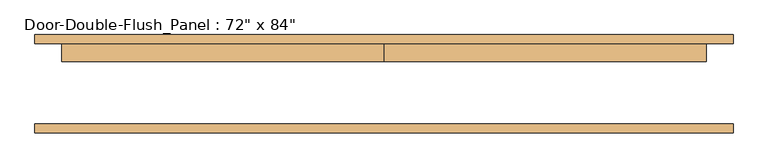
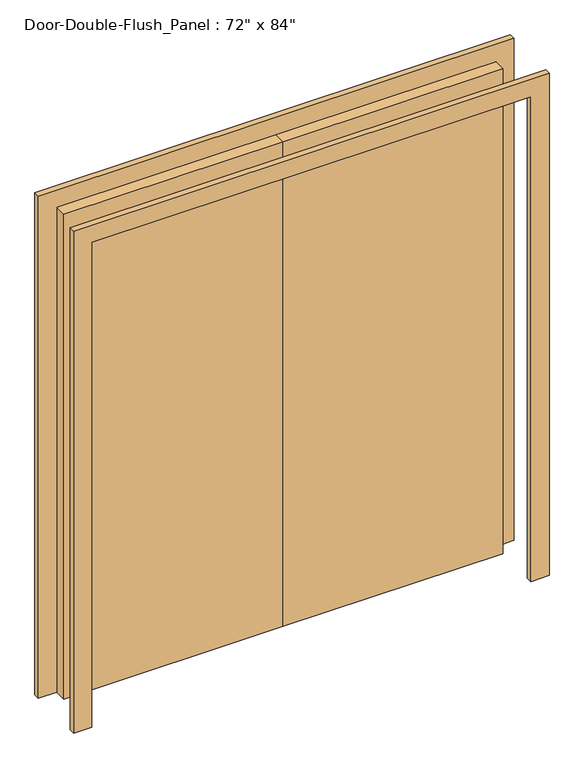
"""IFC4 building model written with IfcOpenShell, lengths in millimetres: door geometry."""

from ifc_helpers import new_model, si_unit, frame, origin, origin_with_axes, place, context, project, spatial, polyline, outline, extrude, source, transform, mapped, element, save


def door_640b4634(model_context):
    return source(origin(), model_context, "Body", "SweptSolid", [
        extrude(outline(polyline([(2133.6, -914.4), (2133.6, 914.4), (0.0, 914.4), (0.0, 990.6), (2209.8, 990.6), (2209.8, -990.6), (0.0, -990.6), (0.0, -914.4), (2133.6, -914.4)])), frame((0.0, -139.7, 0.0), z_axis=(0.0, 1.0, 0.0), x_axis=(0.0, 0.0, 1.0)), (0.0, 0.0, 1.0), 25.4),
        extrude(outline(polyline([(2133.6, -914.4), (2133.6, 914.4), (0.0, 914.4), (0.0, 990.6), (2209.8, 990.6), (2209.8, -990.6), (0.0, -990.6), (0.0, -914.4), (2133.6, -914.4)])), frame((0.0, 114.3, 0.0), z_axis=(0.0, 1.0, 0.0), x_axis=(0.0, 0.0, 1.0)), (0.0, 0.0, 1.0), 25.4),
        extrude(outline(polyline([(0.0, 114.3), (914.4, 114.3), (914.4, 63.5), (0.0, 63.5), (0.0, 114.3)])), origin_with_axes(), (0.0, 0.0, 1.0), 2133.6),
        extrude(outline(polyline([(-914.4, 114.3), (0.0, 114.3), (0.0, 63.5), (-914.4, 63.5), (-914.4, 114.3)])), origin_with_axes(), (0.0, 0.0, 1.0), 2133.6),
    ])


if __name__ == "__main__":
    model = new_model("IFC4")
    model_context = context("Model", 3, world=origin())
    ifc_project = project(units=[si_unit("LENGTHUNIT", "METRE", prefix="MILLI")], contexts=[model_context])
    site = spatial("IfcSite", under=ifc_project)
    building = spatial("IfcBuilding", under=site)
    placement = place(None, origin())
    door_shape = door_640b4634(model_context)
    element("IfcDoor", 1, ObjectType="Door-Double-Flush_Panel : 72\" x 84\"", at=placement, inside=building, context=model_context, shape_type="MappedRepresentation", body=[
        mapped(door_shape, transform((0.0, 0.0, 0.0), x_axis=(1.0, 0.0, 0.0), y_axis=(0.0, 1.0, 0.0), z_axis=(0.0, 0.0, 1.0))),
    ])
    save(model, "model.ifc")

# Revit data of these elements
# Type "Door-Double-Flush_Panel : 72\" x 84\""
#   Type Mark = "11"
#   Construction Type Id = "DOOR"
#   Assembly Code = "C1020"
#   Analytic Construction = "Wooden"
#   Thickness = 0' - 2"
#   Thermal Resistance (R) = 2.5876 (h·ft²·°F)/BTU
#   Swing Angle [instance default] = 90.00°
#   Panel Width = 3' - 0"
#   Heat Transfer Coefficient (U) = 0.3865 BTU/(h·ft²·°F)
#   Height = 7' - 0"
#   Trim Projection Ext = 0' - 1"
#   Trim Projection Int = 0' - 1"
#   Trim Width = 0' - 3"
#   Width = 6' - 0"
#   Define Thermal Properties by = 1
#   Panel Material = Glass, Clear Glazing
#   Trim Material = Paint - Sienna
#   Visual Light Transmittance = 0
#   Solar Heat Gain Coefficient = 0
#   Function = (empty or 0)
#   Wall Closure = (empty or 0)
# Element 1 (IfcDoor, "Door-Double-Flush_Panel : 72\" x 84\"")
#   Materials on its faces: "Paint - Sienna", "Glass, Clear Glazing"
# Materials
#   "Glass, Clear Glazing": class "Glass", colour RGB 0 128 192, transparency 0.75, Description = "Clear glazing", Cost = 0
#   "Paint - Sienna": colour RGB 118 70 51, transparency 0, Cost = 0
